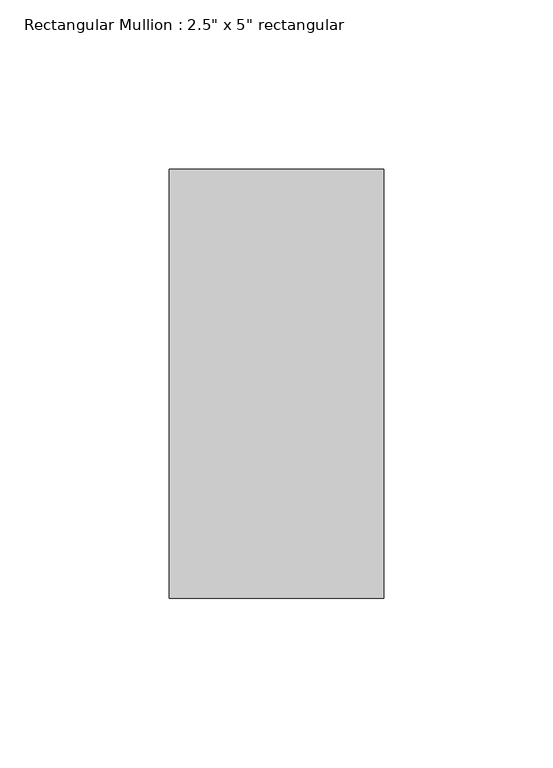
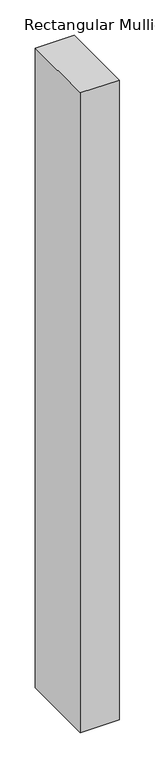
"""IFC4 building model written with IfcOpenShell, lengths in millimetres: member geometry."""

from ifc_helpers import new_model, si_unit, frame, origin, place, context, project, spatial, polyline, outline, extrude, source, transform, mapped, element, save


def member_a8c92c1b(model_context):
    return source(origin(), model_context, "Body", "SweptSolid", [
        extrude(outline(polyline([(0.0, 63.5), (0.0, -63.5), (-63.5, -63.5), (-63.5, 63.5), (0.0, 63.5)])), frame((0.0, 0.0, -1102.7842439), z_axis=(0.0, 0.0, 1.0), x_axis=(1.0, 0.0, 0.0)), (0.0, 0.0, 1.0), 1102.7842439),
    ])


if __name__ == "__main__":
    model = new_model("IFC4")
    model_context = context("Model", 3, world=origin())
    ifc_project = project(units=[si_unit("LENGTHUNIT", "METRE", prefix="MILLI")], contexts=[model_context])
    site = spatial("IfcSite", under=ifc_project)
    building = spatial("IfcBuilding", under=site)
    placement = place(None, origin())
    member_shape = member_a8c92c1b(model_context)
    element("IfcMember", 1, ObjectType="Rectangular Mullion : 2.5\" x 5\" rectangular", at=placement, inside=building, context=model_context, shape_type="MappedRepresentation", body=[
        mapped(member_shape, transform((0.0, 0.0, 0.0), x_axis=(1.0, 0.0, 0.0), y_axis=(0.0, 1.0, 0.0), z_axis=(0.0, 0.0, 1.0))),
    ])
    save(model, "model.ifc")

# Revit data of these elements
# Type "Rectangular Mullion : 2.5\" x 5\" rectangular"
#   built-in parameter 1007304 = 0.416667 (stored number, unit not read)
#   built-in parameter 1007301 = 0.104167 (stored number, unit not read)
#   built-in parameter 1007300 = 0.104167 (stored number, unit not read)
# Element 1 (IfcMember, "Rectangular Mullion : 2.5\" x 5\" rectangular")
#   Materials on its faces: "Aluminum"
# Materials
#   "Aluminum": class "Metal", colour RGB 247 247 247, transparency 0, Description = "Aluminum 6061", Cost = 0
